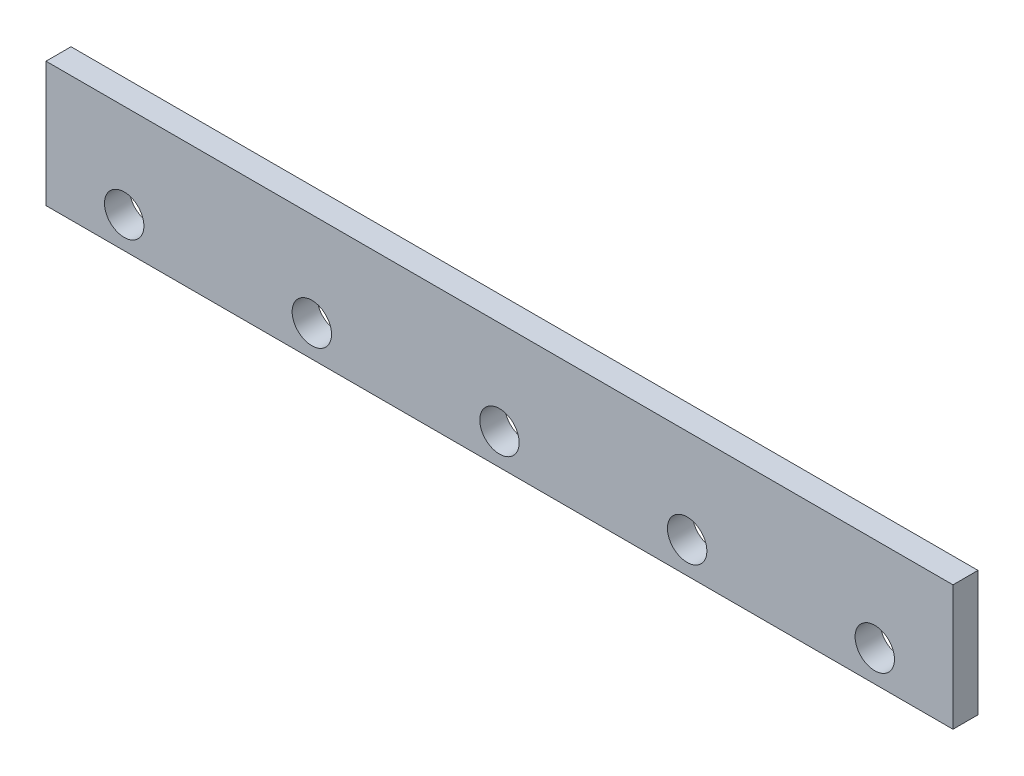
ISO-10303-21;
HEADER;
FILE_DESCRIPTION(('STEP AP214'),'2;1');
FILE_NAME('part.step','',(''),(''),'','','');
FILE_SCHEMA(('AUTOMOTIVE_DESIGN { 1 0 10303 214 1 1 1 1 }'));
ENDSEC;
DATA;
#1=APPLICATION_CONTEXT('core data for automotive mechanical design processes');
#2=APPLICATION_PROTOCOL_DEFINITION('international standard','automotive_design',2000,#1);
#3=PRODUCT_CONTEXT('',#1,'mechanical');
#4=PRODUCT('Part','Part','',(#3));
#5=PRODUCT_RELATED_PRODUCT_CATEGORY('part','',(#4));
#6=PRODUCT_DEFINITION_FORMATION('','',#4);
#7=PRODUCT_DEFINITION_CONTEXT('part definition',#1,'design');
#8=PRODUCT_DEFINITION('design','',#6,#7);
#9=PRODUCT_DEFINITION_SHAPE('','',#8);
#10=(LENGTH_UNIT() NAMED_UNIT(*) SI_UNIT(.MILLI.,.METRE.));
#11=(NAMED_UNIT(*) PLANE_ANGLE_UNIT() SI_UNIT($,.RADIAN.));
#12=(NAMED_UNIT(*) SI_UNIT($,.STERADIAN.) SOLID_ANGLE_UNIT());
#13=UNCERTAINTY_MEASURE_WITH_UNIT(LENGTH_MEASURE(1.E-05),#10,'distance_accuracy_value','');
#14=(GEOMETRIC_REPRESENTATION_CONTEXT(3) GLOBAL_UNCERTAINTY_ASSIGNED_CONTEXT((#13)) GLOBAL_UNIT_ASSIGNED_CONTEXT((#10,
#11,#12)) REPRESENTATION_CONTEXT('',''));
#15=CARTESIAN_POINT('',(0.,0.,0.));
#16=DIRECTION('',(0.,0.,1.));
#17=DIRECTION('',(1.,0.,0.));
#18=AXIS2_PLACEMENT_3D('',#15,#16,#17);
#19=CARTESIAN_POINT('',(290.,40.,16.));
#20=DIRECTION('',(-1.,0.,0.));
#21=DIRECTION('',(0.,0.,1.));
#22=AXIS2_PLACEMENT_3D('',#19,#20,#21);
#23=PLANE('',#22);
#24=DIRECTION('',(0.,1.,0.));
#25=VECTOR('',#24,1.);
#26=CARTESIAN_POINT('',(290.,40.,0.));
#27=LINE('',#26,#25);
#28=CARTESIAN_POINT('',(290.,-40.,0.));
#29=VERTEX_POINT('',#28);
#30=CARTESIAN_POINT('',(290.,40.,0.));
#31=VERTEX_POINT('',#30);
#32=EDGE_CURVE('E105',#29,#31,#27,.T.);
#33=ORIENTED_EDGE('',*,*,#32,.T.);
#34=DIRECTION('',(0.,0.,-1.));
#35=VECTOR('',#34,1.);
#36=CARTESIAN_POINT('',(290.,40.,16.));
#37=LINE('',#36,#35);
#38=CARTESIAN_POINT('',(290.,40.,16.));
#39=VERTEX_POINT('',#38);
#40=EDGE_CURVE('E11',#39,#31,#37,.T.);
#41=ORIENTED_EDGE('',*,*,#40,.F.);
#42=DIRECTION('',(0.,1.,0.));
#43=VECTOR('',#42,1.);
#44=CARTESIAN_POINT('',(290.,40.,16.));
#45=LINE('',#44,#43);
#46=CARTESIAN_POINT('',(290.,-40.,16.));
#47=VERTEX_POINT('',#46);
#48=EDGE_CURVE('E89',#47,#39,#45,.T.);
#49=ORIENTED_EDGE('',*,*,#48,.F.);
#50=DIRECTION('',(0.,0.,-1.));
#51=VECTOR('',#50,1.);
#52=CARTESIAN_POINT('',(290.,-40.,16.));
#53=LINE('',#52,#51);
#54=EDGE_CURVE('E98',#47,#29,#53,.T.);
#55=ORIENTED_EDGE('',*,*,#54,.T.);
#56=EDGE_LOOP('',(#33,#41,#49,#55));
#57=FACE_BOUND('',#56,.T.);
#58=ADVANCED_FACE('F39',(#57),#23,.F.);
#59=CARTESIAN_POINT('',(-290.,40.,16.));
#60=DIRECTION('',(0.,-1.,0.));
#61=DIRECTION('',(0.,0.,-1.));
#62=AXIS2_PLACEMENT_3D('',#59,#60,#61);
#63=PLANE('',#62);
#64=DIRECTION('',(-1.,0.,0.));
#65=VECTOR('',#64,1.);
#66=CARTESIAN_POINT('',(-290.,40.,0.));
#67=LINE('',#66,#65);
#68=CARTESIAN_POINT('',(-290.,40.,0.));
#69=VERTEX_POINT('',#68);
#70=EDGE_CURVE('E94',#31,#69,#67,.T.);
#71=ORIENTED_EDGE('',*,*,#70,.T.);
#72=DIRECTION('',(0.,0.,-1.));
#73=VECTOR('',#72,1.);
#74=CARTESIAN_POINT('',(-290.,40.,16.));
#75=LINE('',#74,#73);
#76=CARTESIAN_POINT('',(-290.,40.,16.));
#77=VERTEX_POINT('',#76);
#78=EDGE_CURVE('E50',#77,#69,#75,.T.);
#79=ORIENTED_EDGE('',*,*,#78,.F.);
#80=DIRECTION('',(-1.,0.,0.));
#81=VECTOR('',#80,1.);
#82=CARTESIAN_POINT('',(-290.,40.,16.));
#83=LINE('',#82,#81);
#84=EDGE_CURVE('E84',#39,#77,#83,.T.);
#85=ORIENTED_EDGE('',*,*,#84,.F.);
#86=ORIENTED_EDGE('',*,*,#40,.T.);
#87=EDGE_LOOP('',(#71,#79,#85,#86));
#88=FACE_BOUND('',#87,.T.);
#89=ADVANCED_FACE('F91',(#88),#63,.F.);
#90=CARTESIAN_POINT('',(-290.,40.,16.));
#91=DIRECTION('',(1.,0.,0.));
#92=DIRECTION('',(0.,0.,-1.));
#93=AXIS2_PLACEMENT_3D('',#90,#91,#92);
#94=PLANE('',#93);
#95=DIRECTION('',(0.,-1.,0.));
#96=VECTOR('',#95,1.);
#97=CARTESIAN_POINT('',(-290.,40.,0.));
#98=LINE('',#97,#96);
#99=CARTESIAN_POINT('',(-290.,-40.,0.));
#100=VERTEX_POINT('',#99);
#101=EDGE_CURVE('E75',#69,#100,#98,.T.);
#102=ORIENTED_EDGE('',*,*,#101,.T.);
#103=DIRECTION('',(0.,0.,-1.));
#104=VECTOR('',#103,1.);
#105=CARTESIAN_POINT('',(-290.,-40.,16.));
#106=LINE('',#105,#104);
#107=CARTESIAN_POINT('',(-290.,-40.,16.));
#108=VERTEX_POINT('',#107);
#109=EDGE_CURVE('E92',#108,#100,#106,.T.);
#110=ORIENTED_EDGE('',*,*,#109,.F.);
#111=DIRECTION('',(0.,-1.,0.));
#112=VECTOR('',#111,1.);
#113=CARTESIAN_POINT('',(-290.,40.,16.));
#114=LINE('',#113,#112);
#115=EDGE_CURVE('E86',#77,#108,#114,.T.);
#116=ORIENTED_EDGE('',*,*,#115,.F.);
#117=ORIENTED_EDGE('',*,*,#78,.T.);
#118=EDGE_LOOP('',(#102,#110,#116,#117));
#119=FACE_BOUND('',#118,.T.);
#120=ADVANCED_FACE('F96',(#119),#94,.F.);
#121=CARTESIAN_POINT('',(-290.,-40.,16.));
#122=DIRECTION('',(0.,1.,0.));
#123=DIRECTION('',(0.,0.,1.));
#124=AXIS2_PLACEMENT_3D('',#121,#122,#123);
#125=PLANE('',#124);
#126=DIRECTION('',(1.,0.,0.));
#127=VECTOR('',#126,1.);
#128=CARTESIAN_POINT('',(-290.,-40.,0.));
#129=LINE('',#128,#127);
#130=EDGE_CURVE('E77',#100,#29,#129,.T.);
#131=ORIENTED_EDGE('',*,*,#130,.T.);
#132=ORIENTED_EDGE('',*,*,#54,.F.);
#133=DIRECTION('',(1.,0.,0.));
#134=VECTOR('',#133,1.);
#135=CARTESIAN_POINT('',(-290.,-40.,16.));
#136=LINE('',#135,#134);
#137=EDGE_CURVE('E54',#108,#47,#136,.T.);
#138=ORIENTED_EDGE('',*,*,#137,.F.);
#139=ORIENTED_EDGE('',*,*,#109,.T.);
#140=EDGE_LOOP('',(#131,#132,#138,#139));
#141=FACE_BOUND('',#140,.T.);
#142=ADVANCED_FACE('F109',(#141),#125,.F.);
#143=CARTESIAN_POINT('',(0.,0.,16.));
#144=DIRECTION('',(0.,0.,1.));
#145=DIRECTION('',(1.,0.,0.));
#146=AXIS2_PLACEMENT_3D('',#143,#144,#145);
#147=PLANE('',#146);
#148=CARTESIAN_POINT('',(-240.,-20.,16.));
#149=DIRECTION('',(0.,0.,1.));
#150=DIRECTION('',(1.,0.,0.));
#151=AXIS2_PLACEMENT_3D('',#148,#149,#150);
#152=CIRCLE('',#151,12.6);
#153=CARTESIAN_POINT('',(-227.4,-20.,16.));
#154=VERTEX_POINT('',#153);
#155=EDGE_CURVE('E139',#154,#154,#152,.T.);
#156=ORIENTED_EDGE('',*,*,#155,.F.);
#157=EDGE_LOOP('',(#156));
#158=FACE_BOUND('',#157,.T.);
#159=CARTESIAN_POINT('',(-120.,-20.,16.));
#160=DIRECTION('',(0.,0.,1.));
#161=DIRECTION('',(1.,0.,0.));
#162=AXIS2_PLACEMENT_3D('',#159,#160,#161);
#163=CIRCLE('',#162,12.6);
#164=CARTESIAN_POINT('',(-107.4,-20.,16.));
#165=VERTEX_POINT('',#164);
#166=EDGE_CURVE('E133',#165,#165,#163,.T.);
#167=ORIENTED_EDGE('',*,*,#166,.F.);
#168=EDGE_LOOP('',(#167));
#169=FACE_BOUND('',#168,.T.);
#170=CARTESIAN_POINT('',(0.,-20.,16.));
#171=DIRECTION('',(0.,0.,1.));
#172=DIRECTION('',(1.,0.,0.));
#173=AXIS2_PLACEMENT_3D('',#170,#171,#172);
#174=CIRCLE('',#173,12.6);
#175=CARTESIAN_POINT('',(12.6000000000001,-20.,16.));
#176=VERTEX_POINT('',#175);
#177=EDGE_CURVE('E126',#176,#176,#174,.T.);
#178=ORIENTED_EDGE('',*,*,#177,.F.);
#179=EDGE_LOOP('',(#178));
#180=FACE_BOUND('',#179,.T.);
#181=CARTESIAN_POINT('',(120.,-20.,16.));
#182=DIRECTION('',(0.,0.,1.));
#183=DIRECTION('',(1.,0.,0.));
#184=AXIS2_PLACEMENT_3D('',#181,#182,#183);
#185=CIRCLE('',#184,12.6);
#186=CARTESIAN_POINT('',(132.6,-20.,16.));
#187=VERTEX_POINT('',#186);
#188=EDGE_CURVE('E125',#187,#187,#185,.T.);
#189=ORIENTED_EDGE('',*,*,#188,.F.);
#190=EDGE_LOOP('',(#189));
#191=FACE_BOUND('',#190,.T.);
#192=CARTESIAN_POINT('',(240.,-20.,16.));
#193=DIRECTION('',(0.,0.,1.));
#194=DIRECTION('',(1.,0.,0.));
#195=AXIS2_PLACEMENT_3D('',#192,#193,#194);
#196=CIRCLE('',#195,12.6);
#197=CARTESIAN_POINT('',(252.6,-20.,16.));
#198=VERTEX_POINT('',#197);
#199=EDGE_CURVE('E116',#198,#198,#196,.T.);
#200=ORIENTED_EDGE('',*,*,#199,.F.);
#201=EDGE_LOOP('',(#200));
#202=FACE_BOUND('',#201,.T.);
#203=ORIENTED_EDGE('',*,*,#48,.T.);
#204=ORIENTED_EDGE('',*,*,#84,.T.);
#205=ORIENTED_EDGE('',*,*,#115,.T.);
#206=ORIENTED_EDGE('',*,*,#137,.T.);
#207=EDGE_LOOP('',(#203,#204,#205,#206));
#208=FACE_BOUND('',#207,.T.);
#209=ADVANCED_FACE('F88',(#158,#169,#180,#191,#202,#208),#147,.T.);
#210=CARTESIAN_POINT('',(0.,0.,0.));
#211=DIRECTION('',(0.,0.,1.));
#212=DIRECTION('',(1.,0.,0.));
#213=AXIS2_PLACEMENT_3D('',#210,#211,#212);
#214=PLANE('',#213);
#215=CARTESIAN_POINT('',(-240.,-20.,0.));
#216=DIRECTION('',(0.,0.,1.));
#217=DIRECTION('',(1.,0.,0.));
#218=AXIS2_PLACEMENT_3D('',#215,#216,#217);
#219=CIRCLE('',#218,12.6);
#220=CARTESIAN_POINT('',(-227.4,-20.,0.));
#221=VERTEX_POINT('',#220);
#222=EDGE_CURVE('E104',#221,#221,#219,.T.);
#223=ORIENTED_EDGE('',*,*,#222,.T.);
#224=EDGE_LOOP('',(#223));
#225=FACE_BOUND('',#224,.T.);
#226=CARTESIAN_POINT('',(-120.,-20.,0.));
#227=DIRECTION('',(0.,0.,1.));
#228=DIRECTION('',(1.,0.,0.));
#229=AXIS2_PLACEMENT_3D('',#226,#227,#228);
#230=CIRCLE('',#229,12.6);
#231=CARTESIAN_POINT('',(-107.4,-20.,0.));
#232=VERTEX_POINT('',#231);
#233=EDGE_CURVE('E140',#232,#232,#230,.T.);
#234=ORIENTED_EDGE('',*,*,#233,.T.);
#235=EDGE_LOOP('',(#234));
#236=FACE_BOUND('',#235,.T.);
#237=CARTESIAN_POINT('',(0.,-20.,0.));
#238=DIRECTION('',(0.,0.,1.));
#239=DIRECTION('',(1.,0.,0.));
#240=AXIS2_PLACEMENT_3D('',#237,#238,#239);
#241=CIRCLE('',#240,12.6);
#242=CARTESIAN_POINT('',(12.6000000000001,-20.,0.));
#243=VERTEX_POINT('',#242);
#244=EDGE_CURVE('E131',#243,#243,#241,.T.);
#245=ORIENTED_EDGE('',*,*,#244,.T.);
#246=EDGE_LOOP('',(#245));
#247=FACE_BOUND('',#246,.T.);
#248=CARTESIAN_POINT('',(120.,-20.,0.));
#249=DIRECTION('',(0.,0.,1.));
#250=DIRECTION('',(1.,0.,0.));
#251=AXIS2_PLACEMENT_3D('',#248,#249,#250);
#252=CIRCLE('',#251,12.6);
#253=CARTESIAN_POINT('',(132.6,-20.,0.));
#254=VERTEX_POINT('',#253);
#255=EDGE_CURVE('E124',#254,#254,#252,.T.);
#256=ORIENTED_EDGE('',*,*,#255,.T.);
#257=EDGE_LOOP('',(#256));
#258=FACE_BOUND('',#257,.T.);
#259=CARTESIAN_POINT('',(240.,-20.,0.));
#260=DIRECTION('',(0.,0.,1.));
#261=DIRECTION('',(1.,0.,0.));
#262=AXIS2_PLACEMENT_3D('',#259,#260,#261);
#263=CIRCLE('',#262,12.6);
#264=CARTESIAN_POINT('',(252.6,-20.,0.));
#265=VERTEX_POINT('',#264);
#266=EDGE_CURVE('E118',#265,#265,#263,.T.);
#267=ORIENTED_EDGE('',*,*,#266,.T.);
#268=EDGE_LOOP('',(#267));
#269=FACE_BOUND('',#268,.T.);
#270=ORIENTED_EDGE('',*,*,#32,.F.);
#271=ORIENTED_EDGE('',*,*,#130,.F.);
#272=ORIENTED_EDGE('',*,*,#101,.F.);
#273=ORIENTED_EDGE('',*,*,#70,.F.);
#274=EDGE_LOOP('',(#270,#271,#272,#273));
#275=FACE_BOUND('',#274,.T.);
#276=ADVANCED_FACE('F114',(#225,#236,#247,#258,#269,#275),#214,.F.);
#277=CARTESIAN_POINT('',(240.,-20.,0.));
#278=DIRECTION('',(0.,0.,1.));
#279=DIRECTION('',(1.,0.,0.));
#280=AXIS2_PLACEMENT_3D('',#277,#278,#279);
#281=CYLINDRICAL_SURFACE('',#280,12.6);
#282=ORIENTED_EDGE('',*,*,#266,.F.);
#283=EDGE_LOOP('',(#282));
#284=FACE_BOUND('',#283,.T.);
#285=ORIENTED_EDGE('',*,*,#199,.T.);
#286=EDGE_LOOP('',(#285));
#287=FACE_BOUND('',#286,.T.);
#288=ADVANCED_FACE('F167',(#284,#287),#281,.F.);
#289=CARTESIAN_POINT('',(120.,-20.,0.));
#290=DIRECTION('',(0.,0.,1.));
#291=DIRECTION('',(1.,0.,0.));
#292=AXIS2_PLACEMENT_3D('',#289,#290,#291);
#293=CYLINDRICAL_SURFACE('',#292,12.6);
#294=ORIENTED_EDGE('',*,*,#255,.F.);
#295=EDGE_LOOP('',(#294));
#296=FACE_BOUND('',#295,.T.);
#297=ORIENTED_EDGE('',*,*,#188,.T.);
#298=EDGE_LOOP('',(#297));
#299=FACE_BOUND('',#298,.T.);
#300=ADVANCED_FACE('F169',(#296,#299),#293,.F.);
#301=CARTESIAN_POINT('',(0.,-20.,0.));
#302=DIRECTION('',(0.,0.,1.));
#303=DIRECTION('',(1.,0.,0.));
#304=AXIS2_PLACEMENT_3D('',#301,#302,#303);
#305=CYLINDRICAL_SURFACE('',#304,12.6);
#306=ORIENTED_EDGE('',*,*,#244,.F.);
#307=EDGE_LOOP('',(#306));
#308=FACE_BOUND('',#307,.T.);
#309=ORIENTED_EDGE('',*,*,#177,.T.);
#310=EDGE_LOOP('',(#309));
#311=FACE_BOUND('',#310,.T.);
#312=ADVANCED_FACE('F174',(#308,#311),#305,.F.);
#313=CARTESIAN_POINT('',(-120.,-20.,0.));
#314=DIRECTION('',(0.,0.,1.));
#315=DIRECTION('',(1.,0.,0.));
#316=AXIS2_PLACEMENT_3D('',#313,#314,#315);
#317=CYLINDRICAL_SURFACE('',#316,12.6);
#318=ORIENTED_EDGE('',*,*,#233,.F.);
#319=EDGE_LOOP('',(#318));
#320=FACE_BOUND('',#319,.T.);
#321=ORIENTED_EDGE('',*,*,#166,.T.);
#322=EDGE_LOOP('',(#321));
#323=FACE_BOUND('',#322,.T.);
#324=ADVANCED_FACE('F151',(#320,#323),#317,.F.);
#325=CARTESIAN_POINT('',(-240.,-20.,0.));
#326=DIRECTION('',(0.,0.,1.));
#327=DIRECTION('',(1.,0.,0.));
#328=AXIS2_PLACEMENT_3D('',#325,#326,#327);
#329=CYLINDRICAL_SURFACE('',#328,12.6);
#330=ORIENTED_EDGE('',*,*,#222,.F.);
#331=EDGE_LOOP('',(#330));
#332=FACE_BOUND('',#331,.T.);
#333=ORIENTED_EDGE('',*,*,#155,.T.);
#334=EDGE_LOOP('',(#333));
#335=FACE_BOUND('',#334,.T.);
#336=ADVANCED_FACE('F146',(#332,#335),#329,.F.);
#337=CLOSED_SHELL('',(#58,#89,#120,#142,#209,#276,#288,#300,#312,#324,#336));
#338=MANIFOLD_SOLID_BREP('B2',#337);
#339=ADVANCED_BREP_SHAPE_REPRESENTATION('',(#18,#338),#14);
#340=SHAPE_DEFINITION_REPRESENTATION(#9,#339);
ENDSEC;
END-ISO-10303-21;
